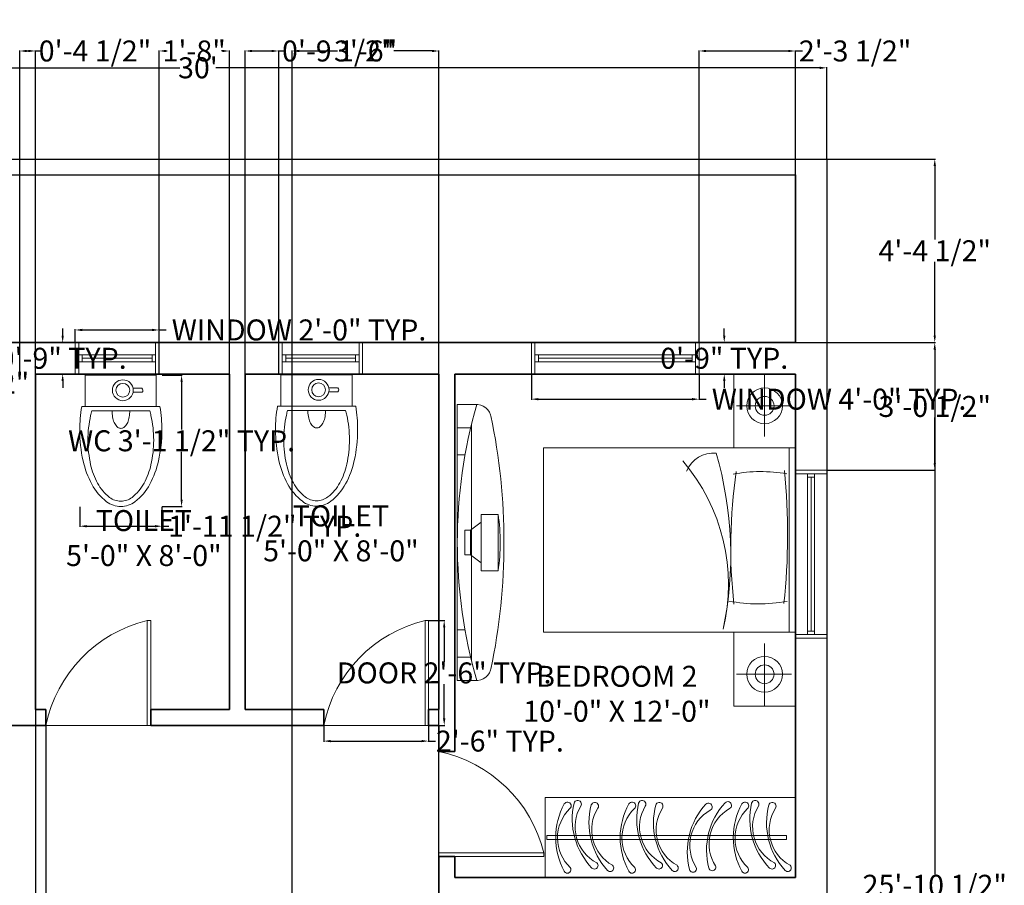
# Model space of a CAD drawing. Units: inches. Extents: x 84 to 590, y 32 to 648.
# Tile 6 of 6: x 262 to 544, y 401 to 648. Entities that reach past the tile are written whole.
import ezdxf

# ---------------------------------------------------------------- set-up
doc = ezdxf.new("R2010")
doc.units = ezdxf.units.IN
doc.header["$MEASUREMENT"] = 0
for name, color, linetype, lineweight in [('A-ANNO-DIMS', 2, 'Continuous', 18), ('A-AREA-IDEN', 7, 'Continuous', 18), ('A-DOOR', 4, 'Continuous', 18), ('A-FLOR-CASE', 9, 'Continuous', 18), ('A-FLOR-FIXT', 9, 'Continuous', 18), ('A-FURN', 8, 'Continuous', 18), ('A-GLAZ', 4, 'Continuous', 18), ('A-WALL', 7, 'Continuous', 35), ('C-PROP', 7, 'Continuous', 30)]:
    doc.layers.add(name, color=color, linetype=linetype, lineweight=lineweight)
doc.styles.get("Standard").update_dxf_attribs({"font": 'arial.ttf'})
doc.dimstyles.get("Standard").update_dxf_attribs({"dimtxt": 6, "dimasz": 2, "dimexe": 0.18, "dimexo": 0.0625, "dimgap": 0.09, "dimtad": 0, "dimtih": 1, "dimtoh": 1, "dimdec": 0, "dimzin": 0, "dimdsep": 46, "dimlunit": 4, "dimtxsty": 'Standard', "dimcen": 0.09, "dimadec": 0, "dimazin": 0, "dimtfac": 1, "dimtdec": 0, "dimtofl": 0, "dimtmove": 0, "dimatfit": 3, "dimfxl": 1, "dimtolj": 1, "dimtzin": 0, "dimarcsym": 1})

# ---------------------------------------------------------------- blocks, each defined once
blk = doc.blocks.new('DOOR')
for p, q in [((185.51, 1128.53), (185.51, 1098.53)), ((185.51, 1128.53), (186.51, 1128.53)), ((186.51, 1098.53), (186.51, 1128.53)), ((186.51, 1098.53), (156.51, 1098.53))]:
    blk.add_line(p, q)
blk.add_arc((194.73, 1090.6), 39.03, 103.6607, 168.2814)
blk = doc.blocks.new('CVBNM')
for p, q in [((388.24, 1592.71), (388.24, 1565.71)), ((420.64, 1592.71), (388.24, 1592.71)), ((420.64, 1592.71), (420.64, 1568.41)), ((420.64, 1482.01), (420.64, 1592.71)), ((501.64, 1592.71), (420.64, 1592.71)), ((420.64, 1565.71), (420.64, 1592.71)), ((501.64, 1592.71), (501.64, 1568.41)), ((501.64, 1592.71), (501.64, 1568.41)), ((501.64, 1482.01), (501.64, 1592.71)), ((501.64, 1565.71), (501.64, 1592.71)), ((501.64, 1592.71), (534.04, 1592.71)), ((534.04, 1592.71), (534.04, 1565.71)), ((402.21, 1579.21), (402.21, 1591.06)), ((501.64, 1590.01), (420.64, 1590.01)), ((520.07, 1579.21), (520.07, 1591.06)), ((402.21, 1579.21), (388.08, 1579.21)), ((402.21, 1579.21), (415.71, 1579.21)), ((402.21, 1579.21), (402.21, 1566.9)), ((520.07, 1579.21), (506.57, 1579.21)), ((520.07, 1579.21), (534.21, 1579.21)), ((520.07, 1579.21), (520.07, 1566.9)), ((388.24, 1565.71), (420.64, 1565.71)), ((534.04, 1565.71), (501.64, 1565.71)), ((501.64, 1482.01), (420.64, 1482.01))]:
    blk.add_line(p, q)
for centre, radius in [((402.21, 1579.21), 7.85), ((402.21, 1579.21), 4.15), ((520.07, 1579.21), 7.85), ((520.07, 1579.21), 4.15)]:
    blk.add_circle(centre, radius)
for centre, radius, start, end in [((458.61, 1300.37), 288.94, 83.953, 95.5626), ((496.51, 1577.48), 65.44, 169.9145, 190.6851), ((419.34, 1576.61), 69.84, 349.1761, 10.2706), ((464.08, 1794.56), 230.23, 261.7649, 276.2896), ((467.83, 1404.8), 159.53, 78.2462, 106.3473), ((480.78, 1479.19), 84.09, 76.5636, 130.3236), ((435.77, 1556.83), 12.88, 175.3269, 247.5588)]:
    blk.add_arc(centre, radius, start, end)
blk = doc.blocks.new('A$C20D7642B')
for p, q in [((0, 1879.7), (0, 0)), ((600, 1879.7), (0, 1879.7)), ((600, 1879.7), (600, 0)), ((285.2, 14), (285.2, 1812.3)), ((285.2, 1812.3), (316, 1812.3)), ((316, 1812.3), (316, 14)), ((340, 0), (0, 0)), ((316, 14), (285.2, 14)), ((340, 0), (600, 0))]:
    blk.add_line(p, q)
for centre, radius, start, end in [((529.2, 1822.6), 26.4, 312.06888, 138.87685), ((189.7, 2189.4), 526.2, 255.30638, 312.74923), ((242.6, 1988.3), 305.1, 237.78554, 330.91711), ((64.5, 1707), 27.8, 56.33784, 252.73759), ((220.7, 1863.8), 305.1, 239.17077, 332.30233), ((511.2, 1705.1), 26.4, 313.4541, 140.26207), ((163, 2063.5), 526.2, 256.69161, 314.13445), ((49.5, 1578.3), 27.8, 57.72306, 254.12281), ((62.8, 1501.9), 27.8, 42.31003, 238.70978), ((303.8, 1731.6), 305.1, 223.75774, 316.8893), ((541.6, 1501.4), 26.4, 298.04107, 124.84904), ((301.2, 1939.5), 526.2, 241.27858, 298.72142), ((59.1, 1372.1), 27.8, 28.28014, 224.67989), ((396.5, 1738.9), 526.2, 227.24868, 284.69153), ((348.6, 1536.6), 305.1, 209.72784, 302.85941), ((523.6, 1255.6), 26.4, 284.01118, 110.81915), ((70.6, 1227.4), 27.8, 28.28014, 224.67989), ((408, 1594.2), 526.2, 227.24868, 284.69153), ((360, 1391.9), 305.1, 209.72784, 302.85941), ((535, 1110.9), 26.4, 284.01118, 110.81915), ((242.6, 1139.3), 305.1, 237.78554, 330.91711), ((529.2, 973.6), 26.4, 312.06888, 138.87685), ((189.7, 1340.3), 526.2, 255.30638, 312.74923), ((64.5, 857.9), 27.8, 56.33784, 252.73759), ((163, 1214.5), 526.2, 256.69161, 314.13445), ((220.7, 1014.8), 305.1, 239.17077, 332.30233), ((511.2, 856), 26.4, 313.4541, 140.26207), ((49.5, 729.2), 27.8, 57.72306, 254.12281), ((62.8, 652.8), 27.8, 42.31003, 238.70978), ((303.8, 882.6), 305.1, 223.75774, 316.8893), ((541.6, 652.4), 26.4, 298.04107, 124.84904), ((301.2, 1090.5), 526.2, 241.27858, 298.72142), ((189.7, 856), 526.2, 255.30638, 312.74923), ((242.6, 655), 305.1, 237.78554, 330.91711), ((529.2, 489.2), 26.4, 312.06888, 138.87685), ((64.5, 373.6), 27.8, 56.33784, 252.73759), ((220.7, 530.5), 305.1, 239.17077, 332.30233), ((511.2, 371.7), 26.4, 313.4541, 140.26207), ((163, 730.2), 526.2, 256.69161, 314.13445), ((49.5, 244.9), 27.8, 57.72306, 254.12281), ((62.8, 168.5), 27.8, 42.31003, 238.70978), ((303.8, 398.3), 305.1, 223.75774, 316.8893), ((541.6, 168), 26.4, 298.04107, 124.84904), ((301.2, 606.1), 526.2, 241.27858, 298.72142)]:
    blk.add_arc(centre, radius, start, end)
blk = doc.blocks.new('A$C78AE5658')
for p, q in [((1515, 306), (1515, 524)), ((1515, 524), (2236, 524)), ((2236, 306), (2236, 524)), ((1515, 306), (2236, 306)), ((1613, 306), (1716, 168)), ((2137, 306), (2034, 168)), ((98, 250), (98, 252)), ((98, 250), (98, 0)), ((348, 184), (3398, 184)), ((398, 0), (398, 172)), ((2034, 168), (1716, 168)), ((1716, 168), (1716, 98)), ((2034, 168), (2034, 98)), ((3348, 0), (3348, 172)), ((3648, 250), (3648, 252)), ((3648, 0), (3648, 250)), ((3648, 0), (98, 0)), ((748, 0), (748, 99)), ((2034, 98), (1716, 98)), ((2998, 0), (2998, 99))]:
    blk.add_line(p, q)
blk.add_lwpolyline([(246, 432, -0.103184), (3500, 432, -0.103184)], format="xyb")
for centre, radius, start, end in [((1875, -1675), 2228, 80.6925, 99.3075), ((298, 239), 200, 98.4687, 183.693), ((3449, 239), 200, 356.307, 81.5313), ((1873, 6426), 6426, 253.9658, 286.0342)]:
    blk.add_arc(centre, radius, start, end)
blk = doc.blocks.new('A$C7FD35E1A')
for p, q in [((0.0233, 0.5799), (0.0233, 0.4408)), ((0.0233, 0.5799), (0.338, 0.5799)), ((0.338, 0.5799), (0.338, 0.4408)), ((0.2356, 0.5044), (0.275, 0.5044)), ((0.2357, 0.5217), (0.2745, 0.5217)), ((0.3542, 0.4408), (0.0087, 0.4408)), ((0.3093, 0.4224), (0.0536, 0.4224))]:
    blk.add_line(p, q)
for radius in [0.046, 0.0305]:
    blk.add_circle((0.1904, 0.5132), radius)
for centre, radius, start, end in [((0.2685, 0.5129), 0.0107, 307.488, 55.394), ((0.6238, 0.337), 0.6238, 170.4184, 180), ((-0.261, 0.337), 0.6238, 0, 9.5816), ((0.5354, 0.2931), 0.4991, 167.4267, 180), ((0.3603, 0.3321), 0.3197, 163.5954, 167.4267), ((0.277, 0.4171), 0.1337, 177.7133, 180), ((0.277, 0.4171), 0.1337, 180, 192.5399), ((0.0869, 0.4171), 0.1337, 347.4601, 0), ((0.0869, 0.4171), 0.1337, 360, 2.2867), ((0.0026, 0.3321), 0.3197, 12.5733, 16.4046), ((-0.1725, 0.2931), 0.4991, 0, 12.5733), ((0.23, 0.4066), 0.0855, 192.5399, 208.2349), ((0.2004, 0.3907), 0.052, 208.2349, 232.3543), ((0.182, 0.3668), 0.0218, 232.3543, 270), ((0.182, 0.3668), 0.0218, 270, 307.6457), ((0.1635, 0.3907), 0.052, 307.6457, 331.7651), ((0.1339, 0.4066), 0.0855, 331.7651, 347.4601), ((0.6238, 0.337), 0.6238, 180, 192.5733), ((-0.261, 0.337), 0.6238, 347.4267, 0), ((0.5354, 0.2931), 0.4991, 180, 192.5733), ((-0.1725, 0.2931), 0.4991, 347.4267, 0), ((0.405, 0.2881), 0.3996, 192.5733, 208.3008), ((0.3603, 0.254), 0.3197, 192.5733, 208.3008), ((0.0026, 0.254), 0.3197, 331.6992, 347.4267), ((-0.0421, 0.2881), 0.3996, 331.6992, 347.4267), ((0.2672, 0.214), 0.2432, 208.3008, 232.4306), ((0.2501, 0.1947), 0.1945, 208.3008, 232.4306), ((0.1128, 0.1947), 0.1945, 307.5694, 331.6992), ((0.0957, 0.214), 0.2432, 307.5694, 331.6992), ((0.1814, 0.1024), 0.1024, 232.4306, 270), ((0.1814, 0.1055), 0.082, 232.4306, 270), ((0.1814, 0.1055), 0.082, 270, 307.5694), ((0.1814, 0.1024), 0.1024, 270, 307.5694)]:
    blk.add_arc(centre, radius, start, end)
blk = doc.blocks.new('*D12')
at = {"layer": 'A-ANNO-DIMS', "color": 0, "lineweight": -2, "transparency": 16777216}
for p, q in [((133.03, 608.4), (133.03, 634.6)), ((135.03, 634.42), (307.85, 634.42)), ((491.03, 634.42), (318.21, 634.42)), ((493.03, 608.4), (493.03, 634.6))]:
    blk.add_line(p, q, dxfattribs=at)
at = {"layer": 'A-ANNO-DIMS', "color": 0, "transparency": 16777216}
for points in [[(135.03, 634.75), (135.03, 634.08), (133.03, 634.42)], [(491.03, 634.75), (491.03, 634.08), (493.03, 634.42)]]:
    blk.add_solid(points, dxfattribs=at)
at = {"layer": 'Defpoints', "color": 0, "transparency": 16777216}
for p in [(493.03, 634.42), (133.03, 608.34), (493.03, 608.34)]:
    blk.add_point(p, dxfattribs=at)
at = {"layer": 'A-ANNO-DIMS', "color": 0, "transparency": 16777216, "insert": (313.03, 634.42), "char_height": 6, "attachment_point": 5}
blk.add_mtext("\\A1;30'", dxfattribs=at)
blk = doc.blocks.new('WIND')
for p, q in [((-51.89, 1021.98), (-99.89, 1021.98)), ((-99.89, 1021.98), (-99.89, 1012.98)), ((-98.89, 1021.98), (-98.89, 1012.98)), ((-52.89, 1012.98), (-52.89, 1021.98)), ((-51.89, 1012.98), (-51.89, 1021.98)), ((-98.89, 1018.48), (-52.89, 1018.48)), ((-97.89, 1018.48), (-97.89, 1016.48)), ((-97.89, 1017.48), (-53.89, 1017.48)), ((-53.89, 1016.48), (-53.89, 1018.48)), ((-98.89, 1016.48), (-52.89, 1016.48)), ((-99.89, 1012.98), (-51.89, 1012.98))]:
    blk.add_line(p, q)
blk = doc.blocks.new('DEFRGTRHYUI')
for p, q in [((222.34, 855.96), (222.34, 864.96)), ((222.34, 864.96), (246.34, 864.96)), ((223.34, 855.96), (223.34, 864.96)), ((245.34, 864.96), (245.34, 855.96)), ((246.34, 864.96), (246.34, 855.96)), ((223.34, 861.46), (245.34, 861.46)), ((224.34, 859.46), (224.34, 861.46)), ((224.34, 860.46), (244.34, 860.46)), ((244.34, 861.46), (244.34, 859.46)), ((223.34, 859.46), (245.34, 859.46)), ((246.34, 855.96), (222.34, 855.96))]:
    blk.add_line(p, q)
blk = doc.blocks.new('*D17')
at = {"layer": 'A-ANNO-DIMS', "color": 0, "lineweight": -2, "transparency": 16777216}
for p, q in [((408.48, 546.78), (408.48, 539.46)), ((456.48, 546.78), (456.48, 539.46)), ((410.48, 539.64), (454.48, 539.64)), ((456.48, 539.64), (458.48, 539.64))]:
    blk.add_line(p, q, dxfattribs=at)
at = {"layer": 'A-ANNO-DIMS', "color": 0, "transparency": 16777216}
for points in [[(410.48, 539.97), (410.48, 539.3), (408.48, 539.64)], [(454.48, 539.97), (454.48, 539.3), (456.48, 539.64)]]:
    blk.add_solid(points, dxfattribs=at)
at = {"layer": 'Defpoints', "color": 0, "transparency": 16777216}
for p in [(408.48, 546.84), (456.48, 546.84), (456.48, 539.64)]:
    blk.add_point(p, dxfattribs=at)
at = {"layer": 'A-ANNO-DIMS', "color": 0, "transparency": 16777216, "insert": (496.54, 539.64), "char_height": 6, "attachment_point": 5}
blk.add_mtext('\\A1;WINDOW 4\'-0" TYP.', dxfattribs=at)
blk = doc.blocks.new('*D18')
at = {"layer": 'A-ANNO-DIMS', "color": 0, "lineweight": -2, "transparency": 16777216}
for p, q in [((463.68, 557.84), (463.68, 559.84)), ((456.55, 555.84), (463.86, 555.84)), ((456.55, 546.84), (463.86, 546.84)), ((463.68, 544.84), (463.68, 542.84))]:
    blk.add_line(p, q, dxfattribs=at)
at = {"layer": 'A-ANNO-DIMS', "color": 0, "transparency": 16777216}
for points in [[(463.35, 557.84), (464.02, 557.84), (463.68, 555.84)], [(463.35, 544.84), (464.02, 544.84), (463.68, 546.84)]]:
    blk.add_solid(points, dxfattribs=at)
at = {"layer": 'Defpoints', "color": 0, "transparency": 16777216}
for p in [(456.48, 555.84), (463.68, 555.84), (456.48, 546.84)]:
    blk.add_point(p, dxfattribs=at)
at = {"layer": 'A-ANNO-DIMS', "color": 0, "transparency": 16777216, "insert": (463.68, 551.34), "char_height": 6, "attachment_point": 5}
blk.add_mtext('\\A1;0\'-9" TYP.', dxfattribs=at)
blk = doc.blocks.new('*D19')
at = {"layer": 'A-ANNO-DIMS', "color": 0, "lineweight": -2, "transparency": 16777216}
for p, q in [((277.93, 555.9), (277.93, 559.62)), ((279.93, 559.44), (299.93, 559.44)), ((301.93, 555.9), (301.93, 559.62)), ((301.93, 559.44), (303.93, 559.44))]:
    blk.add_line(p, q, dxfattribs=at)
at = {"layer": 'A-ANNO-DIMS', "color": 0, "transparency": 16777216}
for points in [[(279.93, 559.77), (279.93, 559.1), (277.93, 559.44)], [(299.93, 559.77), (299.93, 559.1), (301.93, 559.44)]]:
    blk.add_solid(points, dxfattribs=at)
at = {"layer": 'Defpoints', "color": 0, "transparency": 16777216}
for p in [(301.93, 559.44), (277.93, 555.84), (301.93, 555.84)]:
    blk.add_point(p, dxfattribs=at)
at = {"layer": 'A-ANNO-DIMS', "color": 0, "transparency": 16777216, "insert": (341.98, 559.44), "char_height": 6, "attachment_point": 5}
blk.add_mtext('\\A1;WINDOW 2\'-0" TYP.', dxfattribs=at)
blk = doc.blocks.new('*D20')
at = {"layer": 'A-ANNO-DIMS', "color": 0, "lineweight": -2, "transparency": 16777216}
for p, q in [((274.33, 557.84), (274.33, 559.84)), ((277.86, 555.84), (274.15, 555.84)), ((277.86, 546.84), (274.15, 546.84)), ((274.33, 544.84), (274.33, 542.84))]:
    blk.add_line(p, q, dxfattribs=at)
at = {"layer": 'A-ANNO-DIMS', "color": 0, "transparency": 16777216}
for points in [[(273.99, 557.84), (274.66, 557.84), (274.33, 555.84)], [(273.99, 544.84), (274.66, 544.84), (274.33, 546.84)]]:
    blk.add_solid(points, dxfattribs=at)
at = {"layer": 'Defpoints', "color": 0, "transparency": 16777216}
for p in [(274.33, 555.84), (277.93, 555.84), (277.93, 546.84)]:
    blk.add_point(p, dxfattribs=at)
at = {"layer": 'A-ANNO-DIMS', "color": 0, "transparency": 16777216, "insert": (274.33, 551.34), "char_height": 6, "attachment_point": 5}
blk.add_mtext('\\A1;0\'-9" TYP.', dxfattribs=at)
blk = doc.blocks.new('*D21')
at = {"layer": 'A-ANNO-DIMS', "color": 0, "lineweight": -2, "transparency": 16777216}
for p, q in [((379.09, 476.34), (383.71, 476.34)), ((383.53, 474.34), (383.53, 464.53)), ((383.53, 448.34), (383.53, 458.14)), ((379.09, 446.34), (383.71, 446.34))]:
    blk.add_line(p, q, dxfattribs=at)
at = {"layer": 'A-ANNO-DIMS', "color": 0, "transparency": 16777216}
for points in [[(383.19, 474.34), (383.86, 474.34), (383.53, 476.34)], [(383.19, 448.34), (383.86, 448.34), (383.53, 446.34)]]:
    blk.add_solid(points, dxfattribs=at)
at = {"layer": 'Defpoints', "color": 0, "transparency": 16777216}
for p in [(379.03, 476.34), (383.53, 476.34), (379.03, 446.34)]:
    blk.add_point(p, dxfattribs=at)
at = {"layer": 'A-ANNO-DIMS', "color": 0, "transparency": 16777216, "insert": (383.53, 461.34), "char_height": 6, "attachment_point": 5}
blk.add_mtext('\\A1;DOOR 2\'-6" TYP.', dxfattribs=at)
blk = doc.blocks.new('*D22')
at = {"layer": 'A-ANNO-DIMS', "color": 0, "lineweight": -2, "transparency": 16777216}
for p, q in [((349.03, 446.28), (349.03, 441.66)), ((379.03, 446.28), (379.03, 441.66)), ((351.03, 441.84), (377.03, 441.84)), ((379.03, 441.84), (381.03, 441.84))]:
    blk.add_line(p, q, dxfattribs=at)
at = {"layer": 'A-ANNO-DIMS', "color": 0, "transparency": 16777216}
for points in [[(351.03, 442.17), (351.03, 441.5), (349.03, 441.84)], [(377.03, 442.17), (377.03, 441.5), (379.03, 441.84)]]:
    blk.add_solid(points, dxfattribs=at)
at = {"layer": 'Defpoints', "color": 0, "transparency": 16777216}
for p in [(349.03, 446.34), (379.03, 446.34), (379.03, 441.84)]:
    blk.add_point(p, dxfattribs=at)
at = {"layer": 'A-ANNO-DIMS', "color": 0, "transparency": 16777216, "insert": (399.46, 441.84), "char_height": 6, "attachment_point": 5}
blk.add_mtext('\\A1;2\'-6" TYP.', dxfattribs=at)
blk = doc.blocks.new('*D29')
at = {"layer": 'A-ANNO-DIMS', "color": 0, "lineweight": -2, "transparency": 16777216}
for p, q in [((302.79, 546.52), (308.55, 546.52)), ((308.37, 544.52), (308.37, 530.92)), ((308.37, 510.93), (308.37, 524.53)), ((302.79, 508.93), (308.55, 508.93))]:
    blk.add_line(p, q, dxfattribs=at)
at = {"layer": 'A-ANNO-DIMS', "color": 0, "transparency": 16777216}
for points in [[(308.04, 544.52), (308.7, 544.52), (308.37, 546.52)], [(308.04, 510.93), (308.7, 510.93), (308.37, 508.93)]]:
    blk.add_solid(points, dxfattribs=at)
at = {"layer": 'Defpoints', "color": 0, "transparency": 16777216}
for p in [(302.73, 546.52), (308.37, 546.52), (302.73, 508.93)]:
    blk.add_point(p, dxfattribs=at)
at = {"layer": 'A-ANNO-DIMS', "color": 0, "transparency": 16777216, "insert": (308.37, 527.73), "char_height": 6, "attachment_point": 5}
blk.add_mtext('\\A1;WC 3\'-1 1/2" TYP.', dxfattribs=at)
blk = doc.blocks.new('*D30')
at = {"layer": 'A-ANNO-DIMS', "color": 0, "lineweight": -2, "transparency": 16777216}
for p, q in [((279.21, 508.87), (279.21, 503.12)), ((302.73, 508.87), (302.73, 503.12)), ((281.21, 503.3), (300.73, 503.3)), ((302.73, 503.3), (304.73, 503.3))]:
    blk.add_line(p, q, dxfattribs=at)
at = {"layer": 'A-ANNO-DIMS', "color": 0, "transparency": 16777216}
for points in [[(281.21, 503.63), (281.21, 502.96), (279.21, 503.3)], [(300.73, 503.63), (300.73, 502.96), (302.73, 503.3)]]:
    blk.add_solid(points, dxfattribs=at)
at = {"layer": 'Defpoints', "color": 0, "transparency": 16777216}
for p in [(279.21, 508.93), (302.73, 508.93), (302.73, 503.3)]:
    blk.add_point(p, dxfattribs=at)
at = {"layer": 'A-ANNO-DIMS', "color": 0, "transparency": 16777216, "insert": (332.15, 503.3), "char_height": 6, "attachment_point": 5}
blk.add_mtext('\\A1;1\'-11 1/2" TYP.', dxfattribs=at)
blk = doc.blocks.new('*D35')
at = {"layer": 'A-ANNO-DIMS', "color": 0, "lineweight": -2, "transparency": 16777216}
for p, q in [((198.64, 540.41), (198.64, 544.41)), ((200.64, 544.23), (222.55, 544.23)), ((224.55, 540.41), (224.55, 544.41)), ((224.55, 544.23), (226.55, 544.23))]:
    blk.add_line(p, q, dxfattribs=at)
at = {"layer": 'A-ANNO-DIMS', "color": 0, "transparency": 16777216}
for points in [[(200.64, 544.57), (200.64, 543.9), (198.64, 544.23)], [(222.55, 544.57), (222.55, 543.9), (224.55, 544.23)]]:
    blk.add_solid(points, dxfattribs=at)
at = {"layer": 'Defpoints', "color": 0, "transparency": 16777216}
for p in [(224.55, 544.23), (198.64, 540.35), (224.55, 540.35)]:
    blk.add_point(p, dxfattribs=at)
at = {"layer": 'A-ANNO-DIMS', "color": 0, "transparency": 16777216, "insert": (245.55, 544.23), "char_height": 6, "attachment_point": 5}
blk.add_mtext('\\A1;SINK 2\'-2"', dxfattribs=at)
blk = doc.blocks.new('*D43')
at = {"layer": 'A-ANNO-DIMS', "color": 0, "lineweight": -2, "transparency": 16777216}
for p, q in [((493.09, 608.34), (524.11, 608.34)), ((523.93, 606.34), (523.93, 585.28)), ((523.93, 557.84), (523.93, 578.9)), ((484.09, 555.84), (524.11, 555.84))]:
    blk.add_line(p, q, dxfattribs=at)
at = {"layer": 'A-ANNO-DIMS', "color": 0, "transparency": 16777216}
for points in [[(523.59, 606.34), (524.26, 606.34), (523.93, 608.34)], [(523.59, 557.84), (524.26, 557.84), (523.93, 555.84)]]:
    blk.add_solid(points, dxfattribs=at)
at = {"layer": 'Defpoints', "color": 0, "transparency": 16777216}
for p in [(493.03, 608.34), (484.03, 555.84), (523.93, 555.84)]:
    blk.add_point(p, dxfattribs=at)
at = {"layer": 'A-ANNO-DIMS', "color": 0, "transparency": 16777216, "insert": (523.93, 582.09), "char_height": 6, "attachment_point": 5}
blk.add_mtext('\\A1;4\'-4 1/2"', dxfattribs=at)
blk = doc.blocks.new('*D44')
at = {"layer": 'A-ANNO-DIMS', "color": 0, "lineweight": -2, "transparency": 16777216}
for p, q in [((484.09, 555.84), (524.11, 555.84)), ((523.93, 553.84), (523.93, 403.78)), ((523.93, 247.34), (523.93, 397.4)), ((484.09, 245.34), (524.11, 245.34))]:
    blk.add_line(p, q, dxfattribs=at)
at = {"layer": 'A-ANNO-DIMS', "color": 0, "transparency": 16777216}
for points in [[(523.59, 553.84), (524.26, 553.84), (523.93, 555.84)], [(523.59, 247.34), (524.26, 247.34), (523.93, 245.34)]]:
    blk.add_solid(points, dxfattribs=at)
at = {"layer": 'Defpoints', "color": 0, "transparency": 16777216}
for p in [(484.03, 555.84), (484.03, 245.34), (523.93, 245.34)]:
    blk.add_point(p, dxfattribs=at)
at = {"layer": 'A-ANNO-DIMS', "color": 0, "transparency": 16777216, "insert": (523.93, 400.59), "char_height": 6, "attachment_point": 5}
blk.add_mtext('\\A1;25\'-10 1/2"', dxfattribs=at)
blk = doc.blocks.new('*D50')
at = {"layer": 'A-ANNO-DIMS', "color": 0, "lineweight": -2, "transparency": 16777216}
for p, q in [((301.93, 546.9), (301.93, 639.42)), ((303.93, 639.24), (304.19, 639.24)), ((320.03, 639.24), (319.76, 639.24)), ((322.03, 546.9), (322.03, 639.42))]:
    blk.add_line(p, q, dxfattribs=at)
at = {"layer": 'A-ANNO-DIMS', "color": 0, "transparency": 16777216}
for points in [[(303.93, 639.57), (303.93, 638.9), (301.93, 639.24)], [(320.03, 639.57), (320.03, 638.9), (322.03, 639.24)]]:
    blk.add_solid(points, dxfattribs=at)
at = {"layer": 'Defpoints', "color": 0, "transparency": 16777216}
for p in [(322.03, 639.24), (301.93, 546.84), (322.03, 546.84)]:
    blk.add_point(p, dxfattribs=at)
at = {"layer": 'A-ANNO-DIMS', "color": 0, "transparency": 16777216, "insert": (311.98, 639.24), "char_height": 6, "attachment_point": 5}
blk.add_mtext('\\A1;1\'-8"', dxfattribs=at)
blk = doc.blocks.new('*D51')
at = {"layer": 'A-ANNO-DIMS', "color": 0, "lineweight": -2, "transparency": 16777216}
for p, q in [((326.53, 546.9), (326.53, 639.42)), ((328.53, 639.24), (334.16, 639.24)), ((336.16, 546.9), (336.16, 639.42)), ((336.16, 639.24), (338.16, 639.24))]:
    blk.add_line(p, q, dxfattribs=at)
at = {"layer": 'A-ANNO-DIMS', "color": 0, "transparency": 16777216}
for points in [[(328.53, 639.57), (328.53, 638.9), (326.53, 639.24)], [(334.16, 639.57), (334.16, 638.9), (336.16, 639.24)]]:
    blk.add_solid(points, dxfattribs=at)
at = {"layer": 'Defpoints', "color": 0, "transparency": 16777216}
for p in [(336.16, 639.24), (326.53, 546.84), (336.16, 546.84)]:
    blk.add_point(p, dxfattribs=at)
at = {"layer": 'A-ANNO-DIMS', "color": 0, "transparency": 16777216, "insert": (353.22, 639.24), "char_height": 6, "attachment_point": 5}
blk.add_mtext('\\A1;0\'-9 1/2"', dxfattribs=at)
blk = doc.blocks.new('*D52')
at = {"layer": 'A-ANNO-DIMS', "color": 0, "lineweight": -2, "transparency": 16777216}
for p, q in [((456.48, 555.9), (456.48, 639.42)), ((458.48, 639.24), (482.03, 639.24)), ((484.03, 555.9), (484.03, 639.42)), ((484.03, 639.24), (486.03, 639.24))]:
    blk.add_line(p, q, dxfattribs=at)
at = {"layer": 'A-ANNO-DIMS', "color": 0, "transparency": 16777216}
for points in [[(458.48, 639.57), (458.48, 638.9), (456.48, 639.24)], [(482.03, 639.57), (482.03, 638.9), (484.03, 639.24)]]:
    blk.add_solid(points, dxfattribs=at)
at = {"layer": 'Defpoints', "color": 0, "transparency": 16777216}
for p in [(484.03, 639.24), (456.48, 555.84), (484.03, 555.84)]:
    blk.add_point(p, dxfattribs=at)
at = {"layer": 'A-ANNO-DIMS', "color": 0, "transparency": 16777216, "insert": (501.13, 639.24), "char_height": 6, "attachment_point": 5}
blk.add_mtext('\\A1;2\'-3 1/2"', dxfattribs=at)
blk = doc.blocks.new('*D56')
at = {"layer": 'A-ANNO-DIMS', "color": 0, "lineweight": -2, "transparency": 16777216}
for p, q in [((484.09, 555.84), (524.11, 555.84)), ((523.93, 553.84), (523.93, 540.76)), ((523.93, 521.29), (523.93, 534.37)), ((493.09, 519.29), (524.11, 519.29))]:
    blk.add_line(p, q, dxfattribs=at)
at = {"layer": 'A-ANNO-DIMS', "color": 0, "transparency": 16777216}
for points in [[(523.59, 553.84), (524.26, 553.84), (523.93, 555.84)], [(523.59, 521.29), (524.26, 521.29), (523.93, 519.29)]]:
    blk.add_solid(points, dxfattribs=at)
at = {"layer": 'Defpoints', "color": 0, "transparency": 16777216}
for p in [(484.03, 555.84), (523.93, 555.84), (493.03, 519.29)]:
    blk.add_point(p, dxfattribs=at)
at = {"layer": 'A-ANNO-DIMS', "color": 0, "transparency": 16777216, "insert": (523.93, 537.56), "char_height": 6, "attachment_point": 5}
blk.add_mtext('\\A1;3\'-0 1/2"', dxfattribs=at)
blk = doc.blocks.new('*D60')
at = {"layer": 'A-ANNO-DIMS', "color": 0, "lineweight": -2, "transparency": 16777216}
for p, q in [((340.03, 362.4), (340.03, 639.42)), ((342.03, 639.24), (352.97, 639.24)), ((380.03, 639.24), (369.09, 639.24)), ((382.03, 362.4), (382.03, 639.42))]:
    blk.add_line(p, q, dxfattribs=at)
at = {"layer": 'A-ANNO-DIMS', "color": 0, "transparency": 16777216}
for points in [[(342.03, 639.57), (342.03, 638.9), (340.03, 639.24)], [(380.03, 639.57), (380.03, 638.9), (382.03, 639.24)]]:
    blk.add_solid(points, dxfattribs=at)
at = {"layer": 'Defpoints', "color": 0, "transparency": 16777216}
for p in [(382.03, 639.24), (340.03, 362.34), (382.03, 362.34)]:
    blk.add_point(p, dxfattribs=at)
at = {"layer": 'A-ANNO-DIMS', "color": 0, "transparency": 16777216, "insert": (361.03, 639.24), "char_height": 6, "attachment_point": 5}
blk.add_mtext('\\A1;3\'-6"', dxfattribs=at)
blk = doc.blocks.new('*D62')
at = {"layer": 'A-ANNO-DIMS', "color": 0, "lineweight": -2, "transparency": 16777216}
for p, q in [((262.03, 546.9), (262.03, 639.42)), ((264.03, 639.24), (264.53, 639.24)), ((266.53, 546.9), (266.53, 639.42)), ((266.53, 639.24), (268.53, 639.24))]:
    blk.add_line(p, q, dxfattribs=at)
at = {"layer": 'A-ANNO-DIMS', "color": 0, "transparency": 16777216}
for points in [[(264.03, 639.57), (264.03, 638.9), (262.03, 639.24)], [(264.53, 639.57), (264.53, 638.9), (266.53, 639.24)]]:
    blk.add_solid(points, dxfattribs=at)
at = {"layer": 'Defpoints', "color": 0, "transparency": 16777216}
for p in [(266.53, 639.24), (262.03, 546.84), (266.53, 546.84)]:
    blk.add_point(p, dxfattribs=at)
at = {"layer": 'A-ANNO-DIMS', "color": 0, "transparency": 16777216, "insert": (283.58, 639.24), "char_height": 6, "attachment_point": 5}
blk.add_mtext('\\A1;0\'-4 1/2"', dxfattribs=at)
blk = doc.blocks.new('*D63')
at = {"layer": 'A-ANNO-DIMS', "color": 0, "lineweight": -2, "transparency": 16777216}
for p, q in [((266.53, 450.78), (266.53, 73.26)), ((269.53, 450.78), (269.53, 73.26)), ((264.53, 73.44), (262.53, 73.44)), ((271.53, 73.44), (273.53, 73.44))]:
    blk.add_line(p, q, dxfattribs=at)
at = {"layer": 'A-ANNO-DIMS', "color": 0, "transparency": 16777216}
for points in [[(264.53, 73.77), (264.53, 73.1), (266.53, 73.44)], [(271.53, 73.77), (271.53, 73.1), (269.53, 73.44)]]:
    blk.add_solid(points, dxfattribs=at)
at = {"layer": 'Defpoints', "color": 0, "transparency": 16777216}
for p in [(266.53, 450.84), (269.53, 450.84), (269.53, 73.44)]:
    blk.add_point(p, dxfattribs=at)
at = {"layer": 'A-ANNO-DIMS', "color": 0, "transparency": 16777216, "insert": (281.59, 73.44), "char_height": 6, "attachment_point": 5}
blk.add_mtext('\\A1;0\'-3"', dxfattribs=at)

msp = doc.modelspace()

# ---------------------------------------------------------------- linework, layer by layer
at = {"layer": 'A-WALL'}
for p, q in [((142.03, 555.84), (484.03, 555.84)), ((266.53, 450.84), (266.53, 546.84)), ((266.53, 546.84), (322.03, 546.84)), ((322.03, 450.84), (322.03, 546.84)), ((326.53, 450.84), (326.53, 546.84)), ((326.53, 546.84), (382.03, 546.84)), ((382.03, 450.84), (382.03, 546.84)), ((386.53, 546.84), (484.03, 546.84)), ((386.53, 438.84), (386.53, 546.84)), ((484.03, 546.84), (484.03, 402.84)), ((266.53, 450.84), (269.53, 450.84)), ((269.53, 446.34), (269.53, 450.84)), ((299.53, 446.34), (299.53, 450.84)), ((299.53, 450.84), (322.03, 450.84)), ((326.53, 450.84), (349.03, 450.84)), ((349.03, 446.34), (349.03, 450.84)), ((379.03, 446.34), (379.03, 450.84)), ((379.03, 450.84), (382.03, 450.84)), ((142.03, 446.34), (269.53, 446.34)), ((299.53, 446.34), (349.03, 446.34)), ((379.03, 446.34), (382.03, 446.34)), ((382.03, 438.84), (382.03, 446.34)), ((382.03, 438.84), (386.53, 438.84)), ((382.03, 398.34), (382.03, 408.84)), ((382.03, 408.84), (386.53, 408.84)), ((386.53, 402.84), (386.53, 408.84)), ((386.53, 402.84), (484.03, 402.84))]:
    msp.add_line(p, q, dxfattribs=at)
at = {"layer": 'C-PROP'}
for p, q in [((133.03, 608.34), (493.03, 608.34)), ((493.03, 608.34), (493.03, 104.34)), ((142.03, 603.84), (484.03, 603.84)), ((484.03, 603.84), (484.03, 555.84))]:
    msp.add_line(p, q, dxfattribs=at)

# ---------------------------------------------------------------- block references
at = {"layer": 'A-DOOR'}
for p in [(113.02, -652.19), (192.52, -652.19)]:
    msp.add_blockref('DOOR', p, dxfattribs=at)
at = {"layer": 'A-DOOR', "rotation": 270}
msp.add_blockref('DOOR', (-716.5, 595.35), dxfattribs=at)
at = {"layer": 'A-FLOR-CASE', "xscale": 0.0381118678123285, "yscale": 0.0381118678123285, "zscale": 0.0381118678123285, "rotation": 270}
msp.add_blockref('A$C20D7642B', (412.39, 425.71), dxfattribs=at)
at = {"layer": 'A-FLOR-FIXT', "xscale": 64.81477217879883, "yscale": 64.81477217879883, "zscale": 64.81477217879883}
for p in [(279.21, 508.93), (335.24, 509.05)]:
    msp.add_blockref('A$C7FD35E1A', p, dxfattribs=at)
at = {"layer": 'A-FURN', "rotation": 270}
for name, p, xscale, yscale, zscale in [('CVBNM', (-553.6, 799.77), 0.6514848881435277, 0.6514848881435277, 0.6514848881435277), ('A$C78AE5658', (387.28, 540.34), 0.0222542726180731, 0.0222542726180731, 0.0222542726180731)]:
    msp.add_blockref(name, p, dxfattribs=dict(at, xscale=xscale, yscale=yscale, zscale=zscale))
at = {"layer": 'A-GLAZ'}
for name, p in [('DEFRGTRHYUI', (55.59, -309.12)), ('DEFRGTRHYUI', (113.83, -309.12)), ('WIND', (508.38, -466.14))]:
    msp.add_blockref(name, p, dxfattribs=at)
at = {"layer": 'A-GLAZ', "rotation": 270}
msp.add_blockref('WIND', (-528.95, 419.4), dxfattribs=at)

# ---------------------------------------------------------------- texts
at = {"layer": 'A-AREA-IDEN', "char_height": 6, "attachment_point": 1}
for s, width, insert in [('\\pxqc;TOILET\\P5\'-0" X 8\'-0"', 61.8454, (266.65, 507.91)), ('\\pxqc;TOILET\\P5\'-0" X 8\'-0"', 61.8454, (323.05, 509.26)), ('\\pxqc;BEDROOM 2\\P10\'-0" X 12\'-0"', 82.2238, (391.83, 463.37))]:
    msp.add_mtext_dynamic_manual_height_columns(s, width=width, gutter_width=30, heights=[0], dxfattribs=dict(at, insert=insert))

# ---------------------------------------------------------------- dimensions: what is measured, and where the dimension line sits
at = {"layer": 'A-ANNO-DIMS'}
for base, p1, p2, override, picture, middle in [((266.53, 639.24), (262.03, 546.84), (266.53, 546.84), {"dimdec": 1, "dimlfac": 1, "dimrnd": 0, "dimzin": 1, "dimdsep": 46, "dimlunit": 4, "dimfrac": 2}, '*D62', (283.58, 639.24)), ((336.16, 639.24), (326.53, 546.84), (336.16, 546.84), {"dimdec": 1, "dimlfac": 1, "dimrnd": 0, "dimzin": 1, "dimdsep": 46, "dimlunit": 4, "dimfrac": 2}, '*D51', (353.22, 639.24)), ((484.0283, 639.2383), (456.4833, 555.8383), (484.0283, 555.8383), {"dimdec": 1, "dimlfac": 1, "dimrnd": 0, "dimzin": 1, "dimdsep": 46, "dimlunit": 4, "dimfrac": 2}, '*D52', (501.1347, 639.2383)), ((322.03, 639.24), (301.93, 546.84), (322.03, 546.84), {"dimdec": 1, "dimlfac": 1, "dimrnd": 0, "dimzin": 1, "dimdsep": 46, "dimlunit": 4, "dimfrac": 2}, '*D50', (311.98, 639.24)), ((382.03, 639.24), (340.03, 362.34), (382.03, 362.34), {"dimdec": 1, "dimlfac": 1, "dimrnd": 0, "dimzin": 1, "dimdsep": 46, "dimlunit": 4, "dimfrac": 2}, '*D60', (361.03, 639.24)), ((493.03, 634.42), (133.03, 608.34), (493.03, 608.34), {"dimclrd": 0, "dimclre": 0, "dimclrt": 0}, '*D12', (313.03, 634.42)), ((269.53, 73.44), (266.53, 450.84), (269.53, 450.84), {"dimdec": 1, "dimlfac": 1, "dimrnd": 0, "dimzin": 1, "dimdsep": 46, "dimlunit": 4, "dimfrac": 2}, '*D63', (281.59, 73.44))]:
    dim = msp.add_linear_dim(base=base, p1=p1, p2=p2, dimstyle='Standard', override=override, dxfattribs=at)
    dim.commit()
    dim.dimension.update_dxf_attribs({"geometry": picture, "text_midpoint": middle})
for base, p1, p2, picture, middle in [((523.93, 555.84), (493.03, 608.34), (484.03, 555.84), '*D43', (523.93, 582.09)), ((523.93, 245.34), (484.03, 555.84), (484.03, 245.34), '*D44', (523.93, 400.59)), ((523.9283, 555.8383), (493.0283, 519.2899), (484.0283, 555.8383), '*D56', (523.9283, 537.5641))]:
    dim = msp.add_linear_dim(base=base, p1=p1, p2=p2, angle=90, dimstyle='Standard', override={"dimdec": 1, "dimlfac": 1, "dimrnd": 0, "dimzin": 1, "dimdsep": 46, "dimlunit": 4, "dimfrac": 2}, dxfattribs=at)
    dim.commit()
    dim.dimension.update_dxf_attribs({"geometry": picture, "text_midpoint": middle})
for base, p1, p2, text, picture, middle in [((301.93, 559.44), (277.93, 555.84), (301.93, 555.84), 'WINDOW <> TYP.', '*D19', (341.98, 559.44)), ((224.55, 544.23), (198.64, 540.35), (224.55, 540.35), 'SINK <>', '*D35', (245.55, 544.23)), ((456.48, 539.64), (408.48, 546.84), (456.48, 546.84), 'WINDOW <> TYP.', '*D17', (496.54, 539.64)), ((302.73, 503.3), (279.21, 508.93), (302.73, 508.93), '<> TYP.', '*D30', (332.15, 503.3)), ((379.03, 441.84), (349.03, 446.34), (379.03, 446.34), '<> TYP.', '*D22', (399.46, 441.84))]:
    dim = msp.add_linear_dim(base=base, p1=p1, p2=p2, text=text, dimstyle='Standard', override={"dimdec": 1, "dimlfac": 1, "dimrnd": 0, "dimzin": 1, "dimdsep": 46, "dimlunit": 4, "dimfrac": 2}, dxfattribs=at)
    dim.commit()
    dim.dimension.update_dxf_attribs({"geometry": picture, "text_midpoint": middle})
for base, p1, p2, text, picture, middle in [((274.33, 555.84), (277.93, 546.84), (277.93, 555.84), '<> TYP.', '*D20', (274.33, 551.34)), ((463.68, 555.84), (456.48, 546.84), (456.48, 555.84), '<> TYP.', '*D18', (463.68, 551.34)), ((308.37, 546.52), (302.73, 508.93), (302.73, 546.52), 'WC <> TYP.', '*D29', (308.37, 527.73)), ((383.53, 476.34), (379.03, 446.34), (379.03, 476.34), 'DOOR <> TYP.', '*D21', (383.53, 461.34))]:
    dim = msp.add_linear_dim(base=base, p1=p1, p2=p2, angle=90, text=text, dimstyle='Standard', override={"dimdec": 1, "dimlfac": 1, "dimrnd": 0, "dimzin": 1, "dimdsep": 46, "dimlunit": 4, "dimfrac": 2}, dxfattribs=at)
    dim.commit()
    dim.dimension.update_dxf_attribs({"geometry": picture, "text_midpoint": middle})

doc.saveas('drawing.dxf')
